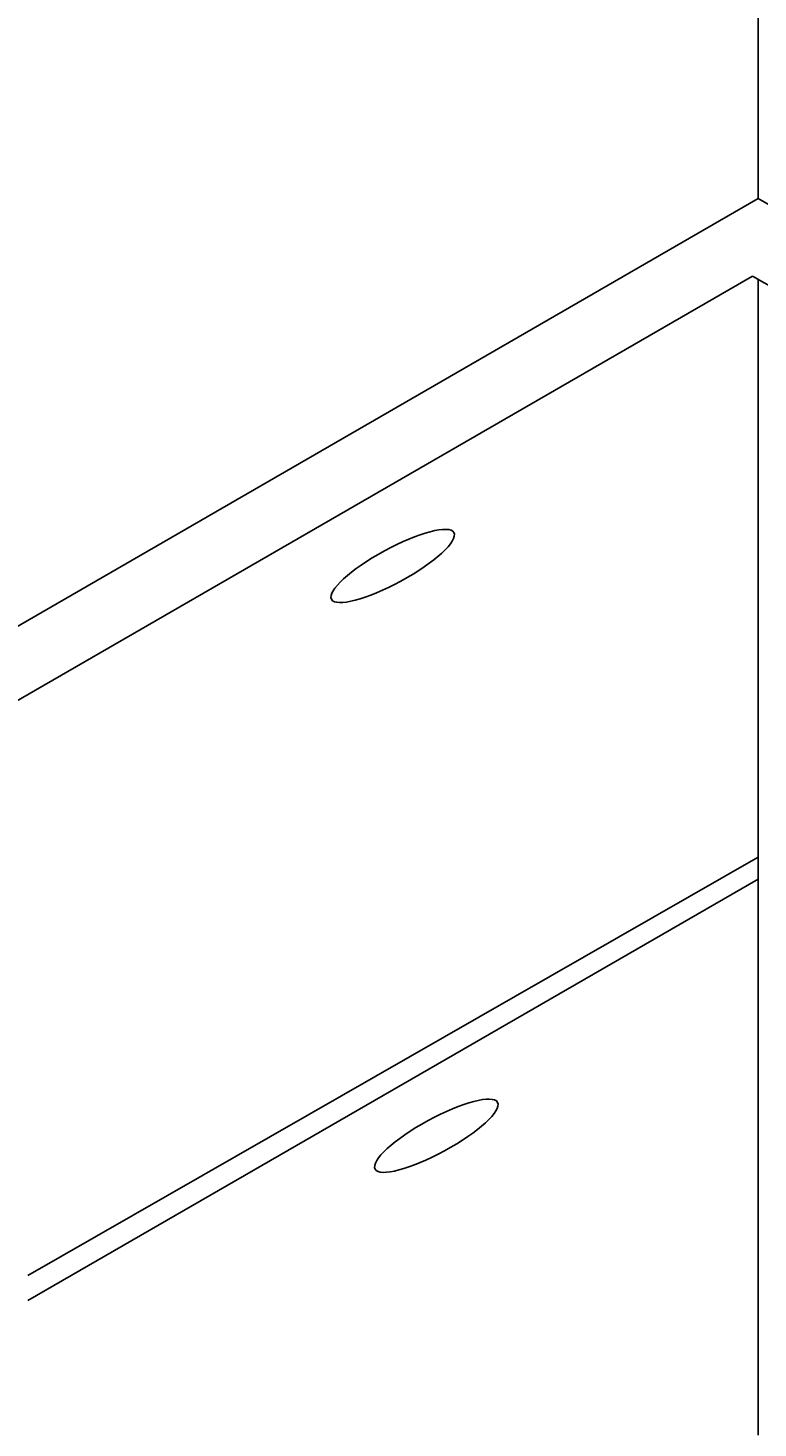
# Model space of a CAD drawing. Units: metres. Extents: x -2391 to 4922, y -635 to 4845.
# Tile 23 of 37: x 31 to 551, y 2130 to 3127. Entities that reach past the tile are written whole.
import ezdxf

# ---------------------------------------------------------------- set-up
doc = ezdxf.new("R2010")
doc.units = ezdxf.units.M
doc.header["$MEASUREMENT"] = 0
doc.layers.add('A-ANNO-DIMS', color=2, linetype='Continuous', lineweight=18)
doc.layers.add('A-FLOR-FIXT', color=3, linetype='Continuous', lineweight=25)
doc.styles.get("Standard").update_dxf_attribs({"font": 'arial.ttf'})
doc.dimstyles.get("Standard").update_dxf_attribs({"dimtxt": 5, "dimasz": 4, "dimexe": 0.18, "dimexo": 0.0625, "dimgap": 0.09, "dimtad": 0, "dimtih": 1, "dimtoh": 1, "dimdec": 0, "dimzin": 0, "dimdsep": 46, "dimtxsty": 'Standard', "dimcen": 0.09, "dimadec": 0, "dimazin": 0, "dimtfac": 1, "dimtdec": 0, "dimtofl": 0, "dimtmove": 0, "dimatfit": 3, "dimfxl": 1, "dimtolj": 1, "dimtzin": 0, "dimarcsym": 0})

# ---------------------------------------------------------------- blocks, each defined once
blk = doc.blocks.new('*D8')
at = {"layer": 'A-ANNO-DIMS', "color": 0, "lineweight": -2, "transparency": 16777216}
for p, q in [((-2047.33, 3005.21), (-2047.33, -631.4)), ((4577.76, 2350.21), (4577.76, -631.4)), ((-2043.33, -631.22), (1257.62, -631.22)), ((4573.76, -631.22), (1272.8, -631.22))]:
    blk.add_line(p, q, dxfattribs=at)
at = {"layer": 'A-ANNO-DIMS', "color": 0, "transparency": 16777216}
for points in [[(-2043.33, -630.56), (-2043.33, -631.89), (-2047.33, -631.22)], [(4573.76, -630.56), (4573.76, -631.89), (4577.76, -631.22)]]:
    blk.add_solid(points, dxfattribs=at)
at = {"layer": 'Defpoints', "color": 0, "transparency": 16777216}
for p in [(-2047.33, 3005.28), (4577.76, 2350.28), (4577.76, -631.22)]:
    blk.add_point(p, dxfattribs=at)
at = {"layer": 'A-ANNO-DIMS', "color": 0, "transparency": 16777216, "insert": (1265.21, -631.22), "char_height": 5, "attachment_point": 5}
blk.add_mtext('\\A1;6625', dxfattribs=at)
blk = doc.blocks.new('*D9')
at = {"layer": 'A-ANNO-DIMS', "color": 0, "lineweight": -2, "transparency": 16777216}
for p, q in [((-2047.33, 3005.34), (-2047.33, 4841.96)), ((-2043.33, 4841.78), (-755.9, 4841.78)), ((546.74, 4841.78), (-740.69, 4841.78)), ((550.74, 4505.34), (550.74, 4841.96))]:
    blk.add_line(p, q, dxfattribs=at)
at = {"layer": 'A-ANNO-DIMS', "color": 0, "transparency": 16777216}
for points in [[(-2043.33, 4842.44), (-2043.33, 4841.11), (-2047.33, 4841.78)], [(546.74, 4842.44), (546.74, 4841.11), (550.74, 4841.78)]]:
    blk.add_solid(points, dxfattribs=at)
at = {"layer": 'Defpoints', "color": 0, "transparency": 16777216}
for p in [(550.74, 4841.78), (550.74, 4505.28), (-2047.33, 3005.28)]:
    blk.add_point(p, dxfattribs=at)
at = {"layer": 'A-ANNO-DIMS', "color": 0, "transparency": 16777216, "insert": (-748.3, 4841.78), "char_height": 5, "attachment_point": 5}
blk.add_mtext('\\A1;2598', dxfattribs=at)
blk = doc.blocks.new('*D10')
at = {"layer": 'A-ANNO-DIMS', "color": 0, "lineweight": -2, "transparency": 16777216}
for p, q in [((550.68, 4505.28), (-2384.01, 4505.28)), ((-2383.83, 4501.28), (-2383.83, 2107.92)), ((-2383.83, -290.72), (-2383.83, 2102.63)), ((-488.55, -294.72), (-2384.01, -294.72))]:
    blk.add_line(p, q, dxfattribs=at)
at = {"layer": 'A-ANNO-DIMS', "color": 0, "transparency": 16777216}
for points in [[(-2384.5, 4501.28), (-2383.17, 4501.28), (-2383.83, 4505.28)], [(-2384.5, -290.72), (-2383.17, -290.72), (-2383.83, -294.72)]]:
    blk.add_solid(points, dxfattribs=at)
at = {"layer": 'Defpoints', "color": 0, "transparency": 16777216}
for p in [(-2383.83, 4505.28), (550.74, 4505.28), (-488.49, -294.72)]:
    blk.add_point(p, dxfattribs=at)
at = {"layer": 'A-ANNO-DIMS', "color": 0, "transparency": 16777216, "insert": (-2383.83, 2105.28), "char_height": 5, "attachment_point": 5}
blk.add_mtext('\\A1;4800', dxfattribs=at)

msp = doc.modelspace()

# ---------------------------------------------------------------- linework, layer by layer
at = {"layer": 'A-FLOR-FIXT'}
for p, q in [((550.7419, 3005.2763), (550.7419, 3684.5146)), ((-228.681, 2555.2763), (550.7419, 3005.2763)), ((550.7419, 3005.2763), (3148.8181, 1505.2763)), ((-182.857, 2528.8198), (546.8938, 2950.1416)), ((546.8938, 2950.1416), (3148.8181, 1447.9199)), ((550.7419, 2947.9199), (550.7419, 2125.2763)), ((31.1266, 2238.8198), (550.7419, 2536.5981)), ((31.1266, 2220.9727), (550.7419, 2520.9727))]:
    msp.add_line(p, q, dxfattribs=at)
for centre in [(290.7251, 2743.8055), (321.7745, 2338.3019)]:
    msp.add_ellipse(centre, major_axis=(43.5598, 23.7449), ratio=0.24668278, dxfattribs=at)

# ---------------------------------------------------------------- dimensions: what is measured, and where the dimension line sits
at = {"layer": 'A-ANNO-DIMS'}
for base, p2, picture, middle in [((550.7419, 4841.7763), (550.7419, 4505.2763), '*D9', (-748.2962, 4841.7763)), ((4577.76, -631.2237), (4577.76, 2350.2763), '*D8', (1265.2128, -631.2237))]:
    dim = msp.add_linear_dim(base=base, p1=(-2047.3343, 3005.2763), p2=p2, dimstyle='Standard', override={"dimdec": 0, "dimlfac": 1, "dimrnd": 0, "dimzin": 0, "dimdsep": 46, "dimlunit": 2}, dxfattribs=at)
    dim.commit()
    dim.dimension.update_dxf_attribs({"geometry": picture, "text_midpoint": middle})
dim = msp.add_linear_dim(base=(-2383.8343, 4505.2763), p1=(-488.4886, -294.7237), p2=(550.7419, 4505.2763), angle=90, dimstyle='Standard', override={"dimdec": 0, "dimlfac": 1, "dimrnd": 0, "dimzin": 0, "dimdsep": 46, "dimlunit": 2}, dxfattribs=at)
dim.commit()
dim.dimension.update_dxf_attribs({"geometry": '*D10', "text_midpoint": (-2383.8343, 2105.2763)})

doc.saveas('drawing.dxf')
